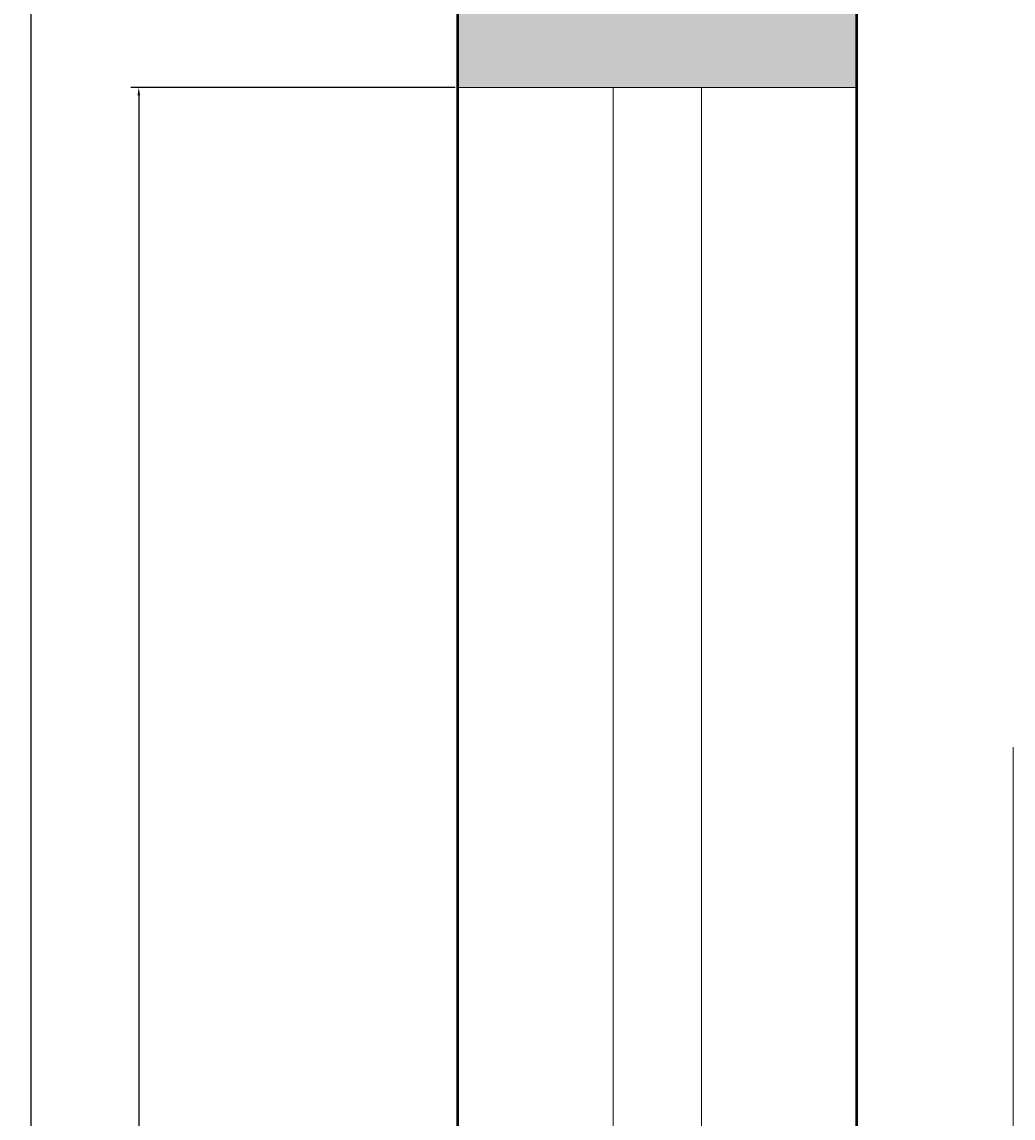
# Model space of a CAD drawing. Units: inches. Extents: x 2231 to 2461, y 2045 to 2455.
# Tile 41 of 95: x 2240 to 2262, y 2247 to 2271. Entities that reach past the tile are written whole.
import ezdxf

# ---------------------------------------------------------------- set-up
doc = ezdxf.new("R2010")
doc.units = ezdxf.units.IN
for name, color, linetype, lineweight in [('A-ANNO-DIMS', 2, 'Continuous', 18), ('A-FURN', 9, 'Continuous', 18), ('A-GLAZ', 4, 'Continuous', 18), ('A-WALL', 7, 'Continuous', 50)]:
    doc.layers.add(name, color=color, linetype=linetype, lineweight=lineweight)
doc.layers.add('A-WALL-PATT', color=18, linetype='Continuous', lineweight=13, true_color=0x000000)
doc.styles.get("Standard").update_dxf_attribs({"font": 'arial.ttf'})
doc.dimstyles.get("Standard").update_dxf_attribs({"dimtxt": 0.18, "dimasz": 0.18, "dimexe": 0.18, "dimexo": 0.0625, "dimgap": 0.09, "dimtad": 0, "dimtih": 1, "dimtoh": 1, "dimdec": 4, "dimzin": 0, "dimdsep": 46, "dimtxsty": 'Standard', "dimcen": 0.09, "dimadec": 0, "dimazin": 0, "dimtfac": 1, "dimtdec": 4, "dimtofl": 0, "dimtmove": 0, "dimatfit": 3, "dimfxl": 1, "dimtolj": 1, "dimtzin": 0, "dimarcsym": 0})

# ---------------------------------------------------------------- blocks, each defined once
blk = doc.blocks.new('WIN-48IN')
for p, q in [((0, 0), (0, 9)), ((48, 9), (48, 0)), ((0, 5.5), (48, 5.5)), ((0, 3.5), (48, 3.5))]:
    blk.add_line(p, q)
blk = doc.blocks.new('*D15')
at = {"layer": 'A-ANNO-DIMS', "color": 0, "lineweight": -2, "transparency": 16777216}
for p, q in [((2249.731, 2269.999), (2242.414, 2269.999)), ((2242.594, 2269.819), (2242.594, 2246.182)), ((2242.594, 2222.179), (2242.594, 2245.816)), ((2249.731, 2221.999), (2242.414, 2221.999))]:
    blk.add_line(p, q, dxfattribs=at)
at = {"layer": 'A-ANNO-DIMS', "color": 0, "transparency": 16777216}
for points in [[(2242.564, 2269.819), (2242.624, 2269.819), (2242.594, 2269.999)], [(2242.564, 2222.179), (2242.624, 2222.179), (2242.594, 2221.999)]]:
    blk.add_solid(points, dxfattribs=at)
at = {"layer": 'Defpoints', "color": 0, "transparency": 16777216}
for p in [(2249.794, 2269.999), (2242.594, 2221.999), (2249.794, 2221.999)]:
    blk.add_point(p, dxfattribs=at)
at = {"layer": 'A-ANNO-DIMS', "color": 0, "transparency": 16777216, "insert": (2242.594, 2245.999), "char_height": 0.18, "attachment_point": 5}
blk.add_mtext('\\A1;WINDOW 48 TYP.', dxfattribs=at)
blk = doc.blocks.new('*D40')
at = {"layer": 'A-ANNO-DIMS', "color": 0, "lineweight": -2, "transparency": 16777216}
for p, q in [((2258.731, 2302.833), (2239.981, 2302.833)), ((2240.161, 2302.653), (2240.161, 2245.015)), ((2240.161, 2187.013), (2240.161, 2244.651)), ((2258.731, 2186.833), (2239.981, 2186.833))]:
    blk.add_line(p, q, dxfattribs=at)
at = {"layer": 'A-ANNO-DIMS', "color": 0, "transparency": 16777216}
for points in [[(2240.131, 2302.653), (2240.191, 2302.653), (2240.161, 2302.833)], [(2240.131, 2187.013), (2240.191, 2187.013), (2240.161, 2186.833)]]:
    blk.add_solid(points, dxfattribs=at)
at = {"layer": 'Defpoints', "color": 0, "transparency": 16777216}
for p in [(2240.161, 2302.833), (2258.794, 2302.833), (2258.794, 2186.833)]:
    blk.add_point(p, dxfattribs=at)
at = {"layer": 'A-ANNO-DIMS', "color": 0, "transparency": 16777216, "insert": (2240.161, 2244.833), "char_height": 0.18, "attachment_point": 5}
blk.add_mtext('\\A1;116', dxfattribs=at)
blk = doc.blocks.new('*D47')
at = {"layer": 'A-ANNO-DIMS', "color": 0, "lineweight": -2, "transparency": 16777216}
for p, q in [((2258.794, 2182.895), (2258.794, 2454.645)), ((2258.974, 2454.465), (2276.575, 2454.465)), ((2294.614, 2454.465), (2277.012, 2454.465)), ((2294.794, 2182.895), (2294.794, 2454.645))]:
    blk.add_line(p, q, dxfattribs=at)
at = {"layer": 'A-ANNO-DIMS', "color": 0, "transparency": 16777216}
for points in [[(2258.974, 2454.495), (2258.974, 2454.435), (2258.794, 2454.465)], [(2294.614, 2454.495), (2294.614, 2454.435), (2294.794, 2454.465)]]:
    blk.add_solid(points, dxfattribs=at)
at = {"layer": 'Defpoints', "color": 0, "transparency": 16777216}
for p in [(2294.794, 2454.465), (2258.794, 2182.833), (2294.794, 2182.833)]:
    blk.add_point(p, dxfattribs=at)
at = {"layer": 'A-ANNO-DIMS', "color": 0, "transparency": 16777216, "insert": (2276.794, 2454.465), "char_height": 0.18, "attachment_point": 5}
blk.add_mtext('\\A1;36', dxfattribs=at)
blk = doc.blocks.new('*D51')
at = {"layer": 'A-ANNO-DIMS', "color": 0, "lineweight": -2, "transparency": 16777216}
for p, q in [((2258.794, 2306.77), (2258.794, 2044.803)), ((2330.794, 2306.77), (2330.794, 2044.803)), ((2258.974, 2044.983), (2294.576, 2044.983)), ((2330.614, 2044.983), (2295.011, 2044.983))]:
    blk.add_line(p, q, dxfattribs=at)
at = {"layer": 'A-ANNO-DIMS', "color": 0, "transparency": 16777216}
for points in [[(2258.974, 2045.013), (2258.974, 2044.953), (2258.794, 2044.983)], [(2330.614, 2045.013), (2330.614, 2044.953), (2330.794, 2044.983)]]:
    blk.add_solid(points, dxfattribs=at)
at = {"layer": 'Defpoints', "color": 0, "transparency": 16777216}
for p in [(2258.794, 2306.833), (2330.794, 2306.833), (2330.794, 2044.983)]:
    blk.add_point(p, dxfattribs=at)
at = {"layer": 'A-ANNO-DIMS', "color": 0, "transparency": 16777216, "insert": (2294.794, 2044.983), "char_height": 0.18, "attachment_point": 5}
blk.add_mtext('\\A1;72', dxfattribs=at)

msp = doc.modelspace()

# ---------------------------------------------------------------- hatches: boundary and pattern name
at = {"layer": 'A-WALL-PATT'}
h = msp.add_hatch(color=256, dxfattribs=at)
h.dxf.hatch_style = 1
h.paths.add_polyline_path([(2441.7935, 2269.1535), (2432.7935, 2269.1535), (2432.7935, 2186.8328), (2396.7935, 2186.8328), (2396.7935, 2286.8328), (2394.7935, 2286.8328), (2394.7935, 2186.8328), (2334.7935, 2186.8328), (2334.7935, 2182.8328), (2432.7935, 2182.8328), (2432.7935, 2072.8328), (2416.6639, 2072.8328), (2416.6639, 2063.8328), (2441.7935, 2063.8328)])
h.paths.add_polyline_path([(2368.6639, 2072.8328), (2367.04, 2072.8328), (2330.7942, 2072.8328), (2330.7397, 2063.8328), (2368.6639, 2063.8328)])
h.paths.add_polyline_path([(2300.7392, 2068.3328), (2300.7392, 2072.8328), (2298.7935, 2072.8328), (2294.7935, 2072.8328), (2258.7935, 2072.8328), (2258.7935, 2120.8328), (2294.7935, 2120.8328), (2298.7935, 2120.8328), (2298.7935, 2128.8328), (2294.7935, 2128.8328), (2294.7935, 2124.8328), (2258.7935, 2124.8328), (2258.7935, 2182.8328), (2294.7935, 2182.8328), (2294.7935, 2174.8328), (2298.7935, 2174.8328), (2298.7935, 2182.8328), (2304.7935, 2182.8328), (2304.7935, 2186.8328), (2258.7935, 2186.8328), (2258.7935, 2221.999), (2249.7935, 2221.999), (2249.7935, 2063.8328), (2300.7392, 2063.8328)])
h.paths.add_polyline_path([(2391.9338, 2435.8328), (2333.82, 2435.8328), (2333.82, 2426.8328), (2368.7935, 2426.8328), (2368.7935, 2374.9508), (2368.7935, 2370.8328), (2372.3935, 2370.8328), (2372.7935, 2370.8328), (2372.7935, 2426.8328), (2391.9338, 2426.8328)])
h.paths.add_polyline_path([(2441.7935, 2435.8328), (2415.9338, 2435.8328), (2415.9338, 2426.8328), (2432.7935, 2426.8328), (2432.7935, 2334.8328), (2372.7935, 2334.8328), (2372.7935, 2346.8328), (2368.7935, 2346.8328), (2368.7935, 2306.8328), (2360.7935, 2306.8328), (2360.7935, 2302.8328), (2368.7935, 2302.8328), (2372.7935, 2302.8328), (2372.7935, 2330.8328), (2432.7935, 2330.8328), (2432.7935, 2317.1535), (2441.7935, 2317.1535)])
h.paths.add_polyline_path([(2285.82, 2435.8328), (2249.7935, 2435.8328), (2249.7935, 2269.999), (2258.7935, 2269.999), (2258.7935, 2302.8328), (2318.8168, 2302.8328), (2330.7935, 2302.8328), (2330.7935, 2306.8328), (2258.7935, 2306.8328), (2258.7935, 2426.8328), (2285.82, 2426.8328)])

# ---------------------------------------------------------------- linework, layer by layer
at = {"layer": 'A-FURN'}
msp.add_line((2262.3207, 2255.1137), (2262.3207, 2195.1137), dxfattribs=at)
at = {"layer": 'A-WALL'}
msp.add_line((2258.7935, 2186.8328), (2258.7935, 2302.8328), dxfattribs=at)
msp.add_lwpolyline([(2300.7392, 2063.8328), (2249.7935, 2063.8328), (2249.7935, 2435.8328), (2441.7935, 2435.8328), (2441.7935, 2063.8328), (2330.7397, 2063.8328)], dxfattribs=at)

# ---------------------------------------------------------------- block references
at = {"layer": 'A-GLAZ', "rotation": 270.000000000001}
msp.add_blockref('WIN-48IN', (2249.7937, 2269.999), dxfattribs=at)

# ---------------------------------------------------------------- dimensions: what is measured, and where the dimension line sits
at = {"layer": 'A-ANNO-DIMS'}
for base, p1, p2, picture, middle in [((2294.7935, 2454.4653), (2258.7935, 2182.8328), (2294.7935, 2182.8328), '*D47', (2276.7935, 2454.4653)), ((2330.7935, 2044.9825), (2258.7935, 2306.8328), (2330.7935, 2306.8328), '*D51', (2294.7935, 2044.9825))]:
    dim = msp.add_linear_dim(base=base, p1=p1, p2=p2, dimstyle='Standard', override={"dimdec": 0, "dimlfac": 1, "dimrnd": 0, "dimzin": 0, "dimdsep": 46, "dimlunit": 2}, dxfattribs=at)
    dim.commit()
    dim.dimension.update_dxf_attribs({"geometry": picture, "text_midpoint": middle})
dim = msp.add_linear_dim(base=(2240.161, 2302.8328), p1=(2258.7935, 2186.8328), p2=(2258.7935, 2302.8328), angle=90, dimstyle='Standard', override={"dimdec": 0, "dimlfac": 1, "dimrnd": 0, "dimzin": 0, "dimdsep": 46, "dimlunit": 2}, dxfattribs=at)
dim.commit()
dim.dimension.update_dxf_attribs({"geometry": '*D40', "text_midpoint": (2240.161, 2244.8328)})
dim = msp.add_linear_dim(base=(2242.5935, 2221.999), p1=(2249.7935, 2269.999), p2=(2249.7935, 2221.999), angle=270, text='WINDOW <> TYP.', dimstyle='Standard', override={"dimdec": 0, "dimlfac": 1, "dimrnd": 0, "dimzin": 0, "dimdsep": 46, "dimlunit": 2}, dxfattribs=at)
dim.commit()
dim.dimension.update_dxf_attribs({"geometry": '*D15', "text_midpoint": (2242.5935, 2245.999)})

doc.saveas('drawing.dxf')
